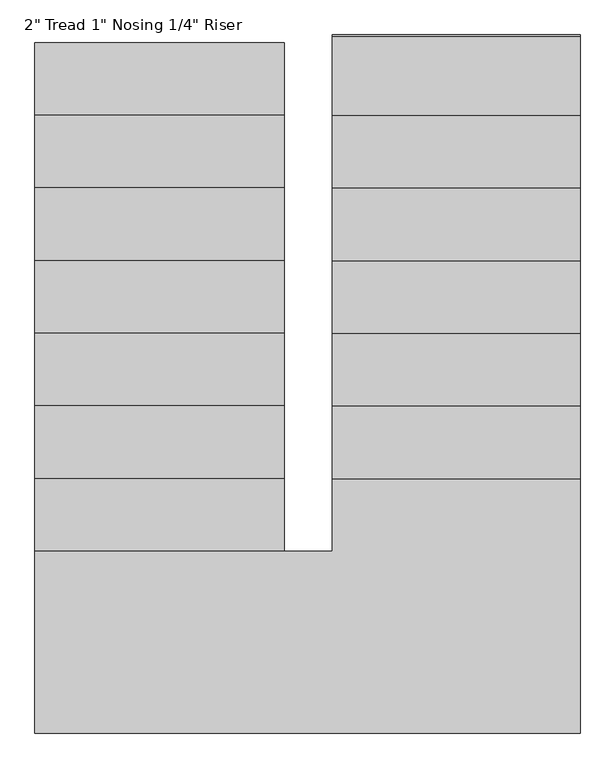
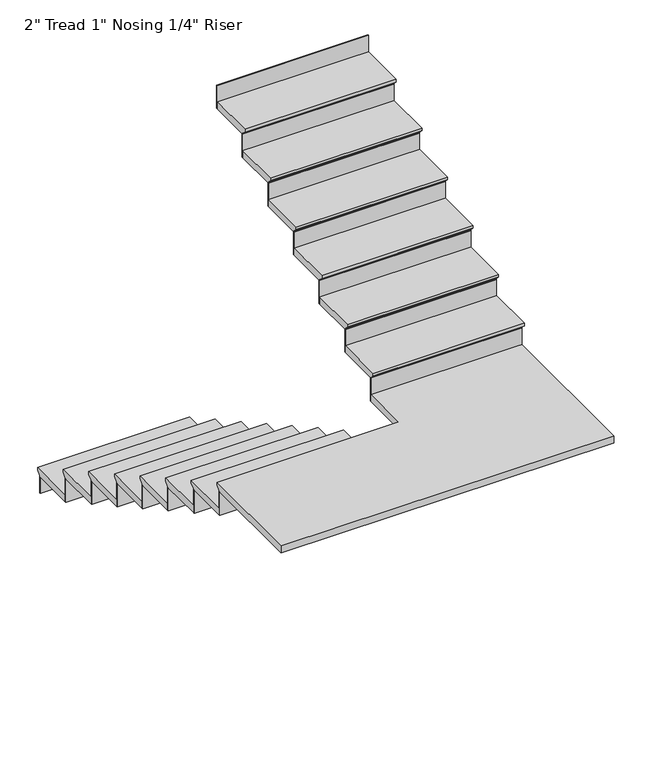
"""IFC4 building model written with IfcOpenShell, lengths in millimetres: stair flight geometry."""

from ifc_helpers import new_model, si_unit, origin, place, context, project, spatial, faceted_brep, source, transform, mapped, element, save


def stair_flight_f50d1433(model_context):
    return source(origin(), model_context, "Body", "Brep", [
        faceted_brep([(-4232.280864, -3571.6080018, 15999.8833333), (-4232.280864, -3571.6080018, 16018.9333333), (-3187.6083919, -3571.6080018, 16018.9333333), (-3187.6083919, -3571.6080018, 15999.8833333), (-4232.280864, -3597.0080018, 15974.4833333), (-3187.6083919, -3597.0080018, 15974.4833333), (-4232.280864, -3901.8080018, 16018.9333333), (-3187.6083919, -3901.8080018, 16018.9333333), (-3187.6083919, -3597.0080018, 15968.1333333), (-3187.6083919, -3901.8080018, 15968.1333333), (-4232.280864, -3901.8080018, 15968.1333333), (-4232.280864, -3597.0080018, 15968.1333333)], [[[0, 1, 2, 3]], [[4, 0, 3, 5]], [[2, 1, 6, 7]], [[8, 9, 10, 11]], [[2, 7, 9, 8, 5, 3]], [[8, 11, 4, 5]], [[6, 1, 0, 4, 11, 10]], [[7, 6, 10, 9]]]),
        faceted_brep([(-4232.280864, -3597.0080018, 15968.1333333), (-4232.280864, -3597.0080018, 15849.6), (-4232.280864, -3603.3580018, 15849.6), (-4232.280864, -3603.3580018, 15968.1333333), (-3187.6083919, -3597.0080018, 15968.1333333), (-3187.6083919, -3603.3580018, 15968.1333333), (-3187.6083919, -3603.3580018, 15849.6), (-3187.6083919, -3597.0080018, 15849.6)], [[[0, 1, 2, 3]], [[4, 5, 6, 7]], [[1, 0, 4, 7]], [[2, 1, 7, 6]], [[3, 2, 6, 5]], [[0, 3, 5, 4]]]),
        faceted_brep([(-4232.280864, -3901.8080018, 16137.4666667), (-4232.280864, -3901.8080018, 15968.1333333), (-4232.280864, -3908.1580018, 15968.1333333), (-4232.280864, -3908.1580018, 16137.4666667), (-3187.6083919, -3901.8080018, 16137.4666667), (-3187.6083919, -3908.1580018, 16137.4666667), (-3187.6083919, -3908.1580018, 15968.1333333), (-3187.6083919, -3901.8080018, 15968.1333333)], [[[0, 1, 2, 3]], [[4, 5, 6, 7]], [[1, 0, 4, 7]], [[2, 1, 7, 6]], [[3, 2, 6, 5]], [[0, 3, 5, 4]]]),
        faceted_brep([(-3187.6083919, -3876.4080018, 16188.2666667), (-4232.280864, -3876.4080018, 16188.2666667), (-4232.280864, -4206.6080018, 16188.2666667), (-3187.6083919, -4206.6080018, 16188.2666667), (-3187.6083919, -3901.8080018, 16137.4666667), (-3187.6083919, -4206.6080018, 16137.4666667), (-4232.280864, -4206.6080018, 16137.4666667), (-4232.280864, -3901.8080018, 16137.4666667), (-3187.6083919, -3901.8080018, 16143.8166667), (-3187.6083919, -3876.4080018, 16169.2166667), (-4232.280864, -3901.8080018, 16143.8166667), (-4232.280864, -3876.4080018, 16169.2166667)], [[[0, 1, 2, 3]], [[4, 5, 6, 7]], [[0, 3, 5, 4, 8, 9]], [[4, 7, 10, 8]], [[2, 1, 11, 10, 7, 6]], [[3, 2, 6, 5]], [[11, 1, 0, 9]], [[10, 11, 9, 8]]]),
        faceted_brep([(-4232.280864, -4206.6080018, 16306.8), (-4232.280864, -4206.6080018, 16137.4666667), (-4232.280864, -4212.9580018, 16137.4666667), (-4232.280864, -4212.9580018, 16306.8), (-3187.6083919, -4206.6080018, 16306.8), (-3187.6083919, -4212.9580018, 16306.8), (-3187.6083919, -4212.9580018, 16137.4666667), (-3187.6083919, -4206.6080018, 16137.4666667)], [[[0, 1, 2, 3]], [[4, 5, 6, 7]], [[1, 0, 4, 7]], [[2, 1, 7, 6]], [[3, 2, 6, 5]], [[0, 3, 5, 4]]]),
        faceted_brep([(-3187.6083919, -4181.2080018, 16357.6), (-4232.280864, -4181.2080018, 16357.6), (-4232.280864, -4511.4080018, 16357.6), (-3187.6083919, -4511.4080018, 16357.6), (-3187.6083919, -4206.6080018, 16306.8), (-3187.6083919, -4511.4080018, 16306.8), (-4232.280864, -4511.4080018, 16306.8), (-4232.280864, -4206.6080018, 16306.8), (-3187.6083919, -4206.6080018, 16313.15), (-3187.6083919, -4181.2080018, 16338.55), (-4232.280864, -4206.6080018, 16313.15), (-4232.280864, -4181.2080018, 16338.55)], [[[0, 1, 2, 3]], [[4, 5, 6, 7]], [[0, 3, 5, 4, 8, 9]], [[4, 7, 10, 8]], [[2, 1, 11, 10, 7, 6]], [[3, 2, 6, 5]], [[11, 1, 0, 9]], [[10, 11, 9, 8]]]),
        faceted_brep([(-4232.280864, -4511.4080018, 16476.1333333), (-4232.280864, -4511.4080018, 16306.8), (-4232.280864, -4517.7580018, 16306.8), (-4232.280864, -4517.7580018, 16476.1333333), (-3187.6083919, -4511.4080018, 16476.1333333), (-3187.6083919, -4517.7580018, 16476.1333333), (-3187.6083919, -4517.7580018, 16306.8), (-3187.6083919, -4511.4080018, 16306.8)], [[[0, 1, 2, 3]], [[4, 5, 6, 7]], [[1, 0, 4, 7]], [[2, 1, 7, 6]], [[3, 2, 6, 5]], [[0, 3, 5, 4]]]),
        faceted_brep([(-3187.6083919, -4486.0080018, 16526.9333333), (-4232.280864, -4486.0080018, 16526.9333333), (-4232.280864, -4816.2080018, 16526.9333333), (-3187.6083919, -4816.2080018, 16526.9333333), (-3187.6083919, -4511.4080018, 16476.1333333), (-3187.6083919, -4816.2080018, 16476.1333333), (-4232.280864, -4816.2080018, 16476.1333333), (-4232.280864, -4511.4080018, 16476.1333333), (-3187.6083919, -4511.4080018, 16482.4833333), (-3187.6083919, -4486.0080018, 16507.8833333), (-4232.280864, -4511.4080018, 16482.4833333), (-4232.280864, -4486.0080018, 16507.8833333)], [[[0, 1, 2, 3]], [[4, 5, 6, 7]], [[0, 3, 5, 4, 8, 9]], [[4, 7, 10, 8]], [[2, 1, 11, 10, 7, 6]], [[3, 2, 6, 5]], [[11, 1, 0, 9]], [[10, 11, 9, 8]]]),
        faceted_brep([(-4232.280864, -4816.2080018, 16645.4666667), (-4232.280864, -4816.2080018, 16476.1333333), (-4232.280864, -4822.5580018, 16476.1333333), (-4232.280864, -4822.5580018, 16645.4666667), (-3187.6083919, -4816.2080018, 16645.4666667), (-3187.6083919, -4822.5580018, 16645.4666667), (-3187.6083919, -4822.5580018, 16476.1333333), (-3187.6083919, -4816.2080018, 16476.1333333)], [[[0, 1, 2, 3]], [[4, 5, 6, 7]], [[1, 0, 4, 7]], [[2, 1, 7, 6]], [[3, 2, 6, 5]], [[0, 3, 5, 4]]]),
        faceted_brep([(-3187.6083919, -4790.8080018, 16696.2666667), (-4232.280864, -4790.8080018, 16696.2666667), (-4232.280864, -5121.0080018, 16696.2666667), (-3187.6083919, -5121.0080018, 16696.2666667), (-3187.6083919, -4816.2080018, 16645.4666667), (-3187.6083919, -5121.0080018, 16645.4666667), (-4232.280864, -5121.0080018, 16645.4666667), (-4232.280864, -4816.2080018, 16645.4666667), (-3187.6083919, -4816.2080018, 16651.8166667), (-3187.6083919, -4790.8080018, 16677.2166667), (-4232.280864, -4816.2080018, 16651.8166667), (-4232.280864, -4790.8080018, 16677.2166667)], [[[0, 1, 2, 3]], [[4, 5, 6, 7]], [[0, 3, 5, 4, 8, 9]], [[4, 7, 10, 8]], [[2, 1, 11, 10, 7, 6]], [[3, 2, 6, 5]], [[11, 1, 0, 9]], [[10, 11, 9, 8]]]),
        faceted_brep([(-4232.280864, -5121.0080018, 16814.8), (-4232.280864, -5121.0080018, 16645.4666667), (-4232.280864, -5127.3580018, 16645.4666667), (-4232.280864, -5127.3580018, 16814.8), (-3187.6083919, -5121.0080018, 16814.8), (-3187.6083919, -5127.3580018, 16814.8), (-3187.6083919, -5127.3580018, 16645.4666667), (-3187.6083919, -5121.0080018, 16645.4666667)], [[[0, 1, 2, 3]], [[4, 5, 6, 7]], [[1, 0, 4, 7]], [[2, 1, 7, 6]], [[3, 2, 6, 5]], [[0, 3, 5, 4]]]),
        faceted_brep([(-3187.6083919, -5095.6080018, 16865.6), (-4232.280864, -5095.6080018, 16865.6), (-4232.280864, -5425.8080018, 16865.6), (-3187.6083919, -5425.8080018, 16865.6), (-3187.6083919, -5121.0080018, 16814.8), (-3187.6083919, -5425.8080018, 16814.8), (-4232.280864, -5425.8080018, 16814.8), (-4232.280864, -5121.0080018, 16814.8), (-3187.6083919, -5121.0080018, 16821.15), (-3187.6083919, -5095.6080018, 16846.55), (-4232.280864, -5121.0080018, 16821.15), (-4232.280864, -5095.6080018, 16846.55)], [[[0, 1, 2, 3]], [[4, 5, 6, 7]], [[0, 3, 5, 4, 8, 9]], [[4, 7, 10, 8]], [[2, 1, 11, 10, 7, 6]], [[3, 2, 6, 5]], [[11, 1, 0, 9]], [[10, 11, 9, 8]]]),
        faceted_brep([(-4232.280864, -5425.8080018, 16984.1333333), (-4232.280864, -5425.8080018, 16814.8), (-4232.280864, -5432.1580018, 16814.8), (-4232.280864, -5432.1580018, 16984.1333333), (-3187.6083919, -5425.8080018, 16984.1333333), (-3187.6083919, -5432.1580018, 16984.1333333), (-3187.6083919, -5432.1580018, 16814.8), (-3187.6083919, -5425.8080018, 16814.8)], [[[0, 1, 2, 3]], [[4, 5, 6, 7]], [[1, 0, 4, 7]], [[2, 1, 7, 6]], [[3, 2, 6, 5]], [[0, 3, 5, 4]]]),
        faceted_brep([(-3187.6083919, -5400.4080018, 17034.9333333), (-4232.280864, -5400.4080018, 17034.9333333), (-4232.280864, -5730.6080018, 17034.9333333), (-3187.6083919, -5730.6080018, 17034.9333333), (-3187.6083919, -5425.8080018, 16984.1333333), (-3187.6083919, -5730.6080018, 16984.1333333), (-4232.280864, -5730.6080018, 16984.1333333), (-4232.280864, -5425.8080018, 16984.1333333), (-3187.6083919, -5425.8080018, 16990.4833333), (-3187.6083919, -5400.4080018, 17015.8833333), (-4232.280864, -5425.8080018, 16990.4833333), (-4232.280864, -5400.4080018, 17015.8833333)], [[[0, 1, 2, 3]], [[4, 5, 6, 7]], [[0, 3, 5, 4, 8, 9]], [[4, 7, 10, 8]], [[2, 1, 11, 10, 7, 6]], [[3, 2, 6, 5]], [[11, 1, 0, 9]], [[10, 11, 9, 8]]]),
        faceted_brep([(-4232.280864, -5730.6080018, 17153.4666667), (-4232.280864, -5730.6080018, 16984.1333333), (-4232.280864, -5736.9580018, 16984.1333333), (-4232.280864, -5736.9580018, 17153.4666667), (-3187.6083919, -5730.6080018, 17153.4666667), (-3187.6083919, -5736.9580018, 17153.4666667), (-3187.6083919, -5736.9580018, 16984.1333333), (-3187.6083919, -5730.6080018, 16984.1333333)], [[[0, 1, 2, 3]], [[4, 5, 6, 7]], [[1, 0, 4, 7]], [[2, 1, 7, 6]], [[3, 2, 6, 5]], [[0, 3, 5, 4]]]),
        faceted_brep([(-2984.4083919, -5375.0080018, 17204.2666667), (-2984.4083919, -5705.2080018, 17204.2666667), (-4232.280864, -5705.2080018, 17204.2666667), (-4232.280864, -6467.2080018, 17204.2666667), (-1946.280864, -6467.2080018, 17204.2666667), (-1946.280864, -5375.0080018, 17204.2666667), (-2984.4083919, -5705.2080018, 17153.4666667), (-2984.4083919, -5375.0080018, 17153.4666667), (-1946.280864, -5375.0080018, 17153.4666667), (-1946.280864, -6467.2080018, 17153.4666667), (-4232.280864, -6467.2080018, 17153.4666667), (-4232.280864, -5730.6080018, 17153.4666667), (-3187.6083919, -5730.6080018, 17153.4666667), (-3187.6083919, -5705.2080018, 17153.4666667), (-3187.6083919, -5705.2080018, 17185.2166667), (-4232.280864, -5705.2080018, 17185.2166667), (-3187.6083919, -5730.6080018, 17159.8166667), (-4232.280864, -5730.6080018, 17159.8166667)], [[[0, 1, 2, 3, 4, 5]], [[6, 7, 8, 9, 10, 11, 12, 13]], [[1, 0, 7, 6]], [[2, 1, 6, 13, 14, 15]], [[13, 12, 16, 14]], [[12, 11, 17, 16]], [[3, 2, 15, 17, 11, 10]], [[4, 3, 10, 9]], [[5, 4, 9, 8]], [[0, 5, 8, 7]], [[17, 15, 14, 16]]]),
        faceted_brep([(-1946.280864, -5375.0080018, 17322.8), (-1946.280864, -5375.0080018, 17153.4666667), (-1946.280864, -5368.6580018, 17153.4666667), (-1946.280864, -5368.6580018, 17322.8), (-2984.4083919, -5375.0080018, 17322.8), (-2984.4083919, -5368.6580018, 17322.8), (-2984.4083919, -5368.6580018, 17153.4666667), (-2984.4083919, -5375.0080018, 17153.4666667)], [[[0, 1, 2, 3]], [[4, 5, 6, 7]], [[1, 0, 4, 7]], [[2, 1, 7, 6]], [[3, 2, 6, 5]], [[0, 3, 5, 4]]]),
        faceted_brep([(-2984.4083919, -5400.4080018, 17373.6), (-1946.280864, -5400.4080018, 17373.6), (-1946.280864, -5070.2080018, 17373.6), (-2984.4083919, -5070.2080018, 17373.6), (-2984.4083919, -5375.0080018, 17322.8), (-2984.4083919, -5070.2080018, 17322.8), (-1946.280864, -5070.2080018, 17322.8), (-1946.280864, -5375.0080018, 17322.8), (-2984.4083919, -5375.0080018, 17329.15), (-2984.4083919, -5400.4080018, 17354.55), (-1946.280864, -5375.0080018, 17329.15), (-1946.280864, -5400.4080018, 17354.55)], [[[0, 1, 2, 3]], [[4, 5, 6, 7]], [[0, 3, 5, 4, 8, 9]], [[4, 7, 10, 8]], [[2, 1, 11, 10, 7, 6]], [[3, 2, 6, 5]], [[11, 1, 0, 9]], [[10, 11, 9, 8]]]),
        faceted_brep([(-1946.280864, -5070.2080018, 17492.1333333), (-1946.280864, -5070.2080018, 17322.8), (-1946.280864, -5063.8580018, 17322.8), (-1946.280864, -5063.8580018, 17492.1333333), (-2984.4083919, -5070.2080018, 17492.1333333), (-2984.4083919, -5063.8580018, 17492.1333333), (-2984.4083919, -5063.8580018, 17322.8), (-2984.4083919, -5070.2080018, 17322.8)], [[[0, 1, 2, 3]], [[4, 5, 6, 7]], [[1, 0, 4, 7]], [[2, 1, 7, 6]], [[3, 2, 6, 5]], [[0, 3, 5, 4]]]),
        faceted_brep([(-2984.4083919, -5095.6080018, 17542.9333333), (-1946.280864, -5095.6080018, 17542.9333333), (-1946.280864, -4765.4080018, 17542.9333333), (-2984.4083919, -4765.4080018, 17542.9333333), (-2984.4083919, -5070.2080018, 17492.1333333), (-2984.4083919, -4765.4080018, 17492.1333333), (-1946.280864, -4765.4080018, 17492.1333333), (-1946.280864, -5070.2080018, 17492.1333333), (-2984.4083919, -5070.2080018, 17498.4833333), (-2984.4083919, -5095.6080018, 17523.8833333), (-1946.280864, -5070.2080018, 17498.4833333), (-1946.280864, -5095.6080018, 17523.8833333)], [[[0, 1, 2, 3]], [[4, 5, 6, 7]], [[0, 3, 5, 4, 8, 9]], [[4, 7, 10, 8]], [[2, 1, 11, 10, 7, 6]], [[3, 2, 6, 5]], [[11, 1, 0, 9]], [[10, 11, 9, 8]]]),
        faceted_brep([(-1946.280864, -4765.4080018, 17661.4666667), (-1946.280864, -4765.4080018, 17492.1333333), (-1946.280864, -4759.0580018, 17492.1333333), (-1946.280864, -4759.0580018, 17661.4666667), (-2984.4083919, -4765.4080018, 17661.4666667), (-2984.4083919, -4759.0580018, 17661.4666667), (-2984.4083919, -4759.0580018, 17492.1333333), (-2984.4083919, -4765.4080018, 17492.1333333)], [[[0, 1, 2, 3]], [[4, 5, 6, 7]], [[1, 0, 4, 7]], [[2, 1, 7, 6]], [[3, 2, 6, 5]], [[0, 3, 5, 4]]]),
        faceted_brep([(-2984.4083919, -4790.8080018, 17712.2666667), (-1946.280864, -4790.8080018, 17712.2666667), (-1946.280864, -4460.6080018, 17712.2666667), (-2984.4083919, -4460.6080018, 17712.2666667), (-2984.4083919, -4765.4080018, 17661.4666667), (-2984.4083919, -4460.6080018, 17661.4666667), (-1946.280864, -4460.6080018, 17661.4666667), (-1946.280864, -4765.4080018, 17661.4666667), (-2984.4083919, -4765.4080018, 17667.8166667), (-2984.4083919, -4790.8080018, 17693.2166667), (-1946.280864, -4765.4080018, 17667.8166667), (-1946.280864, -4790.8080018, 17693.2166667)], [[[0, 1, 2, 3]], [[4, 5, 6, 7]], [[0, 3, 5, 4, 8, 9]], [[4, 7, 10, 8]], [[2, 1, 11, 10, 7, 6]], [[3, 2, 6, 5]], [[11, 1, 0, 9]], [[10, 11, 9, 8]]]),
        faceted_brep([(-1946.280864, -4460.6080018, 17830.8), (-1946.280864, -4460.6080018, 17661.4666667), (-1946.280864, -4454.2580018, 17661.4666667), (-1946.280864, -4454.2580018, 17830.8), (-2984.4083919, -4460.6080018, 17830.8), (-2984.4083919, -4454.2580018, 17830.8), (-2984.4083919, -4454.2580018, 17661.4666667), (-2984.4083919, -4460.6080018, 17661.4666667)], [[[0, 1, 2, 3]], [[4, 5, 6, 7]], [[1, 0, 4, 7]], [[2, 1, 7, 6]], [[3, 2, 6, 5]], [[0, 3, 5, 4]]]),
        faceted_brep([(-2984.4083919, -4486.0080018, 17881.6), (-1946.280864, -4486.0080018, 17881.6), (-1946.280864, -4155.8080018, 17881.6), (-2984.4083919, -4155.8080018, 17881.6), (-2984.4083919, -4460.6080018, 17830.8), (-2984.4083919, -4155.8080018, 17830.8), (-1946.280864, -4155.8080018, 17830.8), (-1946.280864, -4460.6080018, 17830.8), (-2984.4083919, -4460.6080018, 17837.15), (-2984.4083919, -4486.0080018, 17862.55), (-1946.280864, -4460.6080018, 17837.15), (-1946.280864, -4486.0080018, 17862.55)], [[[0, 1, 2, 3]], [[4, 5, 6, 7]], [[0, 3, 5, 4, 8, 9]], [[4, 7, 10, 8]], [[2, 1, 11, 10, 7, 6]], [[3, 2, 6, 5]], [[11, 1, 0, 9]], [[10, 11, 9, 8]]]),
        faceted_brep([(-1946.280864, -4155.8080018, 18000.1333333), (-1946.280864, -4155.8080018, 17830.8), (-1946.280864, -4149.4580018, 17830.8), (-1946.280864, -4149.4580018, 18000.1333333), (-2984.4083919, -4155.8080018, 18000.1333333), (-2984.4083919, -4149.4580018, 18000.1333333), (-2984.4083919, -4149.4580018, 17830.8), (-2984.4083919, -4155.8080018, 17830.8)], [[[0, 1, 2, 3]], [[4, 5, 6, 7]], [[1, 0, 4, 7]], [[2, 1, 7, 6]], [[3, 2, 6, 5]], [[0, 3, 5, 4]]]),
        faceted_brep([(-2984.4083919, -4181.2080018, 18050.9333333), (-1946.280864, -4181.2080018, 18050.9333333), (-1946.280864, -3851.0080018, 18050.9333333), (-2984.4083919, -3851.0080018, 18050.9333333), (-2984.4083919, -4155.8080018, 18000.1333333), (-2984.4083919, -3851.0080018, 18000.1333333), (-1946.280864, -3851.0080018, 18000.1333333), (-1946.280864, -4155.8080018, 18000.1333333), (-2984.4083919, -4155.8080018, 18006.4833333), (-2984.4083919, -4181.2080018, 18031.8833333), (-1946.280864, -4155.8080018, 18006.4833333), (-1946.280864, -4181.2080018, 18031.8833333)], [[[0, 1, 2, 3]], [[4, 5, 6, 7]], [[0, 3, 5, 4, 8, 9]], [[4, 7, 10, 8]], [[2, 1, 11, 10, 7, 6]], [[3, 2, 6, 5]], [[11, 1, 0, 9]], [[10, 11, 9, 8]]]),
        faceted_brep([(-1946.280864, -3851.0080018, 18169.4666667), (-1946.280864, -3851.0080018, 18000.1333333), (-1946.280864, -3844.6580018, 18000.1333333), (-1946.280864, -3844.6580018, 18169.4666667), (-2984.4083919, -3851.0080018, 18169.4666667), (-2984.4083919, -3844.6580018, 18169.4666667), (-2984.4083919, -3844.6580018, 18000.1333333), (-2984.4083919, -3851.0080018, 18000.1333333)], [[[0, 1, 2, 3]], [[4, 5, 6, 7]], [[1, 0, 4, 7]], [[2, 1, 7, 6]], [[3, 2, 6, 5]], [[0, 3, 5, 4]]]),
        faceted_brep([(-1946.280864, -3546.2080018, 18338.8), (-1946.280864, -3546.2080018, 18169.4666667), (-1946.280864, -3539.8580018, 18169.4666667), (-1946.280864, -3539.8580018, 18338.8), (-2984.4083919, -3546.2080018, 18338.8), (-2984.4083919, -3539.8580018, 18338.8), (-2984.4083919, -3539.8580018, 18169.4666667), (-2984.4083919, -3546.2080018, 18169.4666667)], [[[0, 1, 2, 3]], [[4, 5, 6, 7]], [[1, 0, 4, 7]], [[2, 1, 7, 6]], [[3, 2, 6, 5]], [[0, 3, 5, 4]]]),
        faceted_brep([(-2984.4083919, -3876.4080018, 18220.2666667), (-1946.280864, -3876.4080018, 18220.2666667), (-1946.280864, -3546.2080018, 18220.2666667), (-2984.4083919, -3546.2080018, 18220.2666667), (-2984.4083919, -3851.0080018, 18169.4666667), (-2984.4083919, -3546.2080018, 18169.4666667), (-1946.280864, -3546.2080018, 18169.4666667), (-1946.280864, -3851.0080018, 18169.4666667), (-2984.4083919, -3851.0080018, 18175.8166667), (-2984.4083919, -3876.4080018, 18201.2166667), (-1946.280864, -3851.0080018, 18175.8166667), (-1946.280864, -3876.4080018, 18201.2166667)], [[[0, 1, 2, 3]], [[4, 5, 6, 7]], [[0, 3, 5, 4, 8, 9]], [[4, 7, 10, 8]], [[2, 1, 11, 10, 7, 6]], [[3, 2, 6, 5]], [[11, 1, 0, 9]], [[10, 11, 9, 8]]]),
    ])


if __name__ == "__main__":
    model = new_model("IFC4")
    model_context = context("Model", 3, world=origin())
    ifc_project = project(units=[si_unit("LENGTHUNIT", "METRE", prefix="MILLI")], contexts=[model_context])
    site = spatial("IfcSite", under=ifc_project)
    building = spatial("IfcBuilding", under=site)
    placement = place(None, origin())
    stair_flight_shape = stair_flight_f50d1433(model_context)
    element("IfcStairFlight", 1, ObjectType="2\" Tread 1\" Nosing 1/4\" Riser", at=placement, inside=building, context=model_context, shape_type="MappedRepresentation", body=[
        mapped(stair_flight_shape, transform((0.0, 0.0, 0.0), x_axis=(1.0, 0.0, 0.0), y_axis=(0.0, 1.0, 0.0), z_axis=(0.0, 0.0, 1.0))),
    ])
    save(model, "model.ifc")
